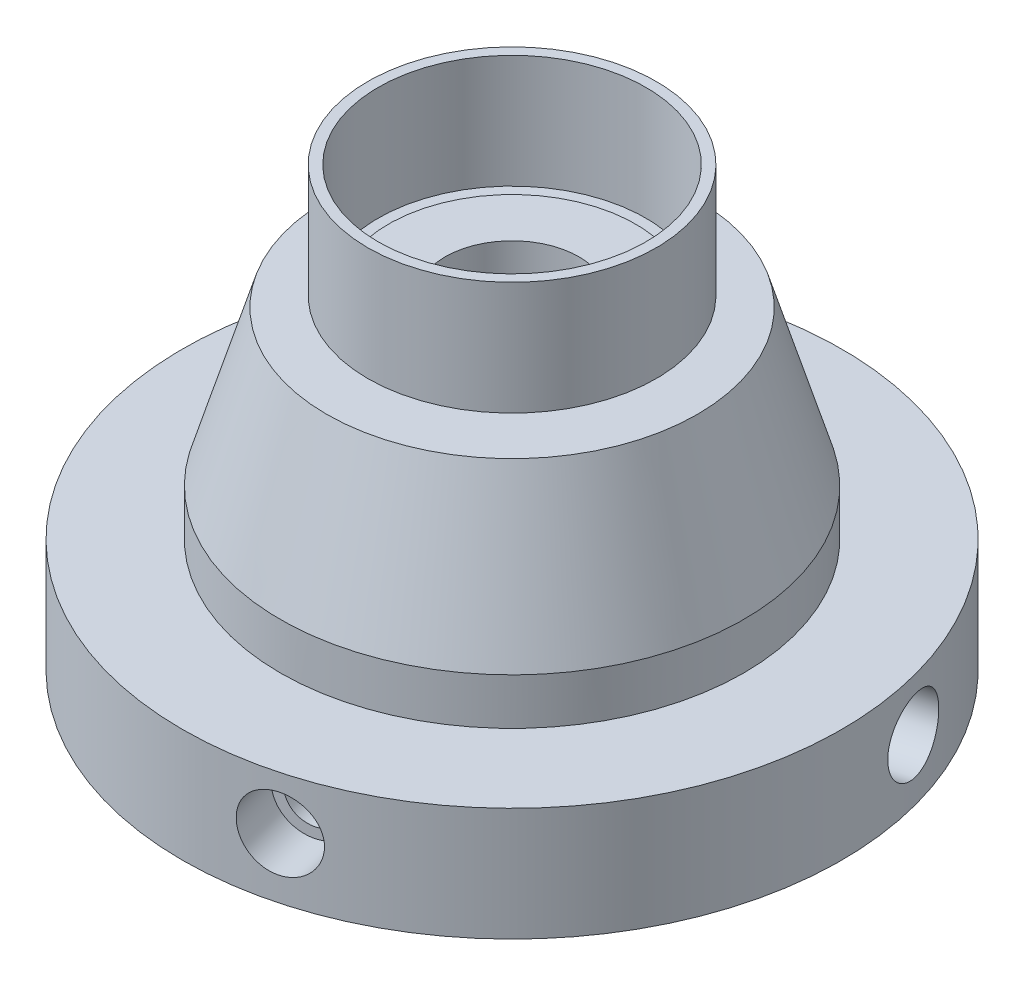
from build123d import *

# Parameters (mm, degrees)
BASE_FLANGE_SKETCH_R          = 64
BASE_FLANGE_128_DEPTH         = 22
COLLAR_SKETCH_R               = 45
COLLAR_90_DEPTH               = 9
LOFT_BASE_PROFILE_R           = 45
LOFT_TOP_PROFILE_72_R         = 36
TOP_STEP_SKETCH_R             = 24
TOP_STEP_48_DEPTH             = 2
TUBE_SKETCH_R                 = 28
TUBE_SKETCH_R_2               = 26
TUBE_56X_52_DEPTH             = 22
RADIAL_HOLES_PATTERN_4X_COUNT = 4
BOTTOM_RECESS_SKETCH_R        = 31
BOTTOM_RECESS_62_DEPTH        = 6
BOTTOM_SLOT_CUT_DEPTH         = 57


with BuildPart() as part:
    # Base Flange Sketch → Base Flange Ø128 (new body)
    with BuildSketch(Plane(origin=(0, 0, 0), x_dir=(1, 0, 0), z_dir=(0, 1, 0))):
        with Locations(Location((0, 0, 0), (0, 0, 270))):
            Circle(BASE_FLANGE_SKETCH_R)
    extrude(amount=BASE_FLANGE_128_DEPTH)

    # Collar Sketch → Collar Ø90 (add)
    with BuildSketch(Plane(origin=(0, 22, 0), x_dir=(1, 0, 0), z_dir=(0, 1, 0))):
        with Locations(Location((0, 0, 0), (0, 0, 270))):
            Circle(COLLAR_SKETCH_R)
    extrude(amount=COLLAR_90_DEPTH)

    # Loft Base Profile → Conical Transition Loft section 0
    with BuildSketch(Plane(origin=(0, 31, 0), x_dir=(1, 0, 0), z_dir=(0, 1, 0))):
        Circle(LOFT_BASE_PROFILE_R)
    # Loft Top Profile Ø72 → Conical Transition Loft section 1
    with BuildSketch(Plane(origin=(0, 61, 0), x_dir=(1, 0, 0), z_dir=(0, 1, 0))):
        Circle(LOFT_TOP_PROFILE_72_R)
    loft()

    # Top Step Sketch → Top Step Ø48 (add)
    with BuildSketch(Plane(origin=(0, 61, 0), x_dir=(1, 0, 0), z_dir=(0, 1, 0))):
        with Locations(Location((0, 0, 0), (0, 0, 270))):
            Circle(TOP_STEP_SKETCH_R)
    extrude(amount=TOP_STEP_48_DEPTH)

    # Sketch15 → Radial C-Bore Hole Ø10 (revolve, cut)
    with BuildSketch(Plane(origin=(61.822507432, 11.6871388, -16.552267966), x_dir=(-0.2586291869671418, 0, -0.9659766786256878), z_dir=(0, 1, 0))):
        Polygon((0, 0), (0, 45), (5, 45), (5, 10), (7, 10), (7, 0), align=None)
    radial_c_bore_hole_10 = revolve(axis=Axis((-44.434927217, 11.6871388, 11.8969426), (0.9659766786256878, 0, -0.25862918696714177)), mode=Mode.SUBTRACT)

    # Radial Holes Pattern 4x: Radial C-Bore Hole Ø10 ×4 about axis
    radial_holes_pattern_4x_axis = Axis((0, 0, 0), (0, 1, 0))
    for i in range(1, RADIAL_HOLES_PATTERN_4X_COUNT):
        add(radial_c_bore_hole_10.rotate(radial_holes_pattern_4x_axis, i * 360 / RADIAL_HOLES_PATTERN_4X_COUNT), mode=Mode.SUBTRACT)

    # Bottom Recess Sketch → Bottom Recess Ø62 (cut)
    with BuildSketch(Plane.XZ):
        with Locations(Location((0, 0, 0), (0, 0, 270))):
            Circle(BOTTOM_RECESS_SKETCH_R)
    extrude(amount=-BOTTOM_RECESS_62_DEPTH, mode=Mode.SUBTRACT)

    # Bottom Slot Sketch → Bottom Slot Cut (cut)
    with BuildSketch(Plane.XZ.offset(-6)):
        with BuildLine():
            Line((12.757350822, 2.5), (16, 2.5))
            Line((16, 2.5), (16, -2.5))
            Line((16, -2.5), (12.757350822, -2.5))
            ThreePointArc((12.757350822, -2.5), (-13, 0), (12.757350822, 2.5))
        make_face()
    extrude(amount=-BOTTOM_SLOT_CUT_DEPTH, mode=Mode.SUBTRACT)


with BuildPart() as body_2:
    # Tube Sketch → Tube Ø56xØ52 (new body)
    with BuildSketch(Plane(origin=(0, 63, 0), x_dir=(1, 0, 0), z_dir=(0, 1, 0))):
        with Locations(Location((0, 0, 0), (0, 0, 270))):
            Circle(TUBE_SKETCH_R)
        with Locations(Location((0, 0, 0), (0, 0, 270))):
            Circle(TUBE_SKETCH_R_2, mode=Mode.SUBTRACT)
    extrude(amount=TUBE_56X_52_DEPTH)


solid = Compound([part.part, body_2.part])
